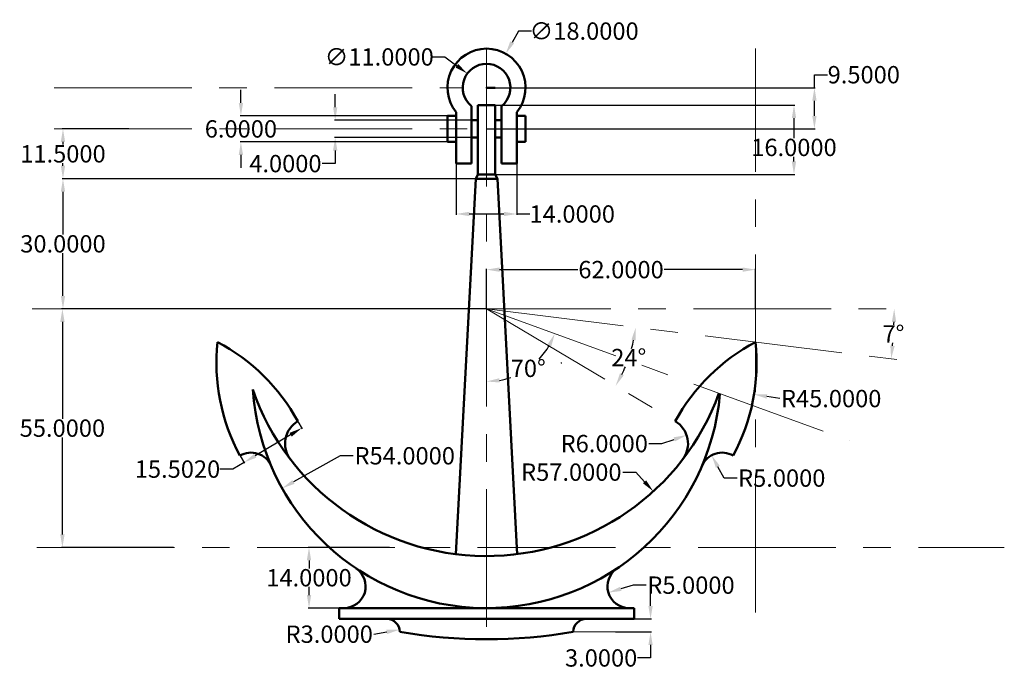
# Model space of a CAD drawing. Units: millimetres. Extents: x 434 to 661, y 625 to 775.
import ezdxf

# ---------------------------------------------------------------- set-up
doc = ezdxf.new("R2010")
doc.units = ezdxf.units.MM
doc.header["$MEASUREMENT"] = 0
doc.linetypes.add('CENTER', pattern=[50.8, 31.75, -6.35, 6.35, -6.35])
for name, color, linetype, lineweight in [('M-CNTR', 1, 'CENTER', 18), ('M-DIMS', 2, 'Continuous', 25), ('M-OUTL', 7, 'Continuous', 50)]:
    doc.layers.add(name, color=color, linetype=linetype, lineweight=lineweight)
doc.styles.get("Standard").update_dxf_attribs({"font": 'arial.ttf'})
doc.dimstyles.get("Standard").update_dxf_attribs({"dimtxt": 4, "dimasz": 3, "dimexe": 0.18, "dimexo": 0.0625, "dimgap": 0.09, "dimtad": 0, "dimtih": 1, "dimtoh": 1, "dimdec": 4, "dimzin": 0, "dimdsep": 46, "dimtxsty": 'Standard', "dimcen": 0.09, "dimadec": 0, "dimazin": 0, "dimtfac": 1, "dimtdec": 4, "dimtofl": 0, "dimtmove": 0, "dimatfit": 3, "dimfxl": 1, "dimtolj": 1, "dimtzin": 0, "dimarcsym": 0})

# ---------------------------------------------------------------- blocks, each defined once
blk = doc.blocks.new('*D1')
at = {"layer": 'Defpoints', "color": 0, "transparency": 16777216}
for p in [(558.86, 696.06), (603.27, 688.77)]:
    blk.add_point(p, dxfattribs=at)
at = {"layer": 'M-DIMS', "color": 0, "lineweight": -2, "transparency": 16777216}
for p, q in [((558.77, 696.06), (558.95, 696.06)), ((558.86, 695.97), (558.86, 696.15)), ((609.19, 687.8), (606.23, 688.28))]:
    blk.add_line(p, q, dxfattribs=at)
at = {"layer": 'M-DIMS', "color": 0, "transparency": 16777216}
blk.add_solid([(606.31, 688.78), (606.14, 687.79), (603.27, 688.77)], dxfattribs=at)
at = {"layer": 'M-DIMS', "color": 0, "transparency": 16777216, "insert": (621.04, 687.8), "char_height": 4, "attachment_point": 5}
blk.add_mtext('\\A1;R45.0000', dxfattribs=at)
blk = doc.blocks.new('*D2')
at = {"layer": 'Defpoints', "color": 0, "transparency": 16777216}
for p in [(593.47, 674.73), (595.87, 670.34)]:
    blk.add_point(p, dxfattribs=at)
at = {"layer": 'M-DIMS', "color": 0, "lineweight": -2, "transparency": 16777216}
for p, q in [((596.35, 669.47), (594.91, 672.1)), ((599.35, 669.47), (596.35, 669.47))]:
    blk.add_line(p, q, dxfattribs=at)
at = {"layer": 'M-DIMS', "color": 0, "transparency": 16777216}
blk.add_solid([(595.35, 672.34), (594.47, 671.86), (593.47, 674.73)], dxfattribs=at)
at = {"layer": 'M-DIMS', "color": 0, "transparency": 16777216, "insert": (609.65, 669.47), "char_height": 4, "attachment_point": 5}
blk.add_mtext('\\A1;R5.0000', dxfattribs=at)
blk = doc.blocks.new('*D3')
at = {"layer": 'Defpoints', "color": 0, "transparency": 16777216}
for p in [(587.72, 679.37), (582.04, 677.42)]:
    blk.add_point(p, dxfattribs=at)
at = {"layer": 'M-DIMS', "color": 0, "lineweight": -2, "transparency": 16777216}
for p, q in [((579.04, 677.42), (582.04, 677.42)), ((582.04, 677.42), (584.88, 678.39))]:
    blk.add_line(p, q, dxfattribs=at)
at = {"layer": 'M-DIMS', "color": 0, "transparency": 16777216}
blk.add_solid([(584.72, 678.87), (585.04, 677.92), (587.72, 679.37)], dxfattribs=at)
at = {"layer": 'M-DIMS', "color": 0, "transparency": 16777216, "insert": (568.74, 677.42), "char_height": 4, "attachment_point": 5}
blk.add_mtext('\\A1;R6.0000', dxfattribs=at)
blk = doc.blocks.new('*D4')
at = {"layer": 'Defpoints', "color": 0, "transparency": 16777216}
for p in [(541.61, 708.49), (580.05, 666.41)]:
    blk.add_point(p, dxfattribs=at)
at = {"layer": 'M-DIMS', "color": 0, "lineweight": -2, "transparency": 16777216}
for p, q in [((573, 670.84), (576, 670.84)), ((576, 670.84), (578.02, 668.62))]:
    blk.add_line(p, q, dxfattribs=at)
at = {"layer": 'M-DIMS', "color": 0, "transparency": 16777216}
blk.add_solid([(578.39, 668.96), (577.65, 668.28), (580.05, 666.41)], dxfattribs=at)
at = {"layer": 'M-DIMS', "color": 0, "transparency": 16777216, "insert": (561.15, 670.84), "char_height": 4, "attachment_point": 5}
blk.add_mtext('\\A1;R57.0000', dxfattribs=at)
blk = doc.blocks.new('*D5')
at = {"layer": 'Defpoints', "color": 0, "transparency": 16777216}
for p in [(541.61, 693.49), (494.49, 667.11)]:
    blk.add_point(p, dxfattribs=at)
at = {"layer": 'M-DIMS', "color": 0, "lineweight": -2, "transparency": 16777216}
for p, q in [((507.89, 674.61), (497.11, 668.57)), ((510.89, 674.61), (507.89, 674.61))]:
    blk.add_line(p, q, dxfattribs=at)
at = {"layer": 'M-DIMS', "color": 0, "transparency": 16777216}
blk.add_solid([(496.86, 669.01), (497.35, 668.14), (494.49, 667.11)], dxfattribs=at)
at = {"layer": 'M-DIMS', "color": 0, "transparency": 16777216, "insert": (522.75, 674.61), "char_height": 4, "attachment_point": 5}
blk.add_mtext('\\A1;R54.0000', dxfattribs=at)
blk = doc.blocks.new('*D6')
at = {"layer": 'Defpoints', "color": 0, "transparency": 16777216}
for p in [(569.68, 643.05), (574.47, 644.49)]:
    blk.add_point(p, dxfattribs=at)
at = {"layer": 'M-DIMS', "color": 0, "lineweight": -2, "transparency": 16777216}
for p, q in [((575.43, 644.78), (572.55, 643.92)), ((578.43, 644.78), (575.43, 644.78))]:
    blk.add_line(p, q, dxfattribs=at)
at = {"layer": 'M-DIMS', "color": 0, "transparency": 16777216}
blk.add_solid([(572.41, 644.4), (572.7, 643.44), (569.68, 643.05)], dxfattribs=at)
at = {"layer": 'M-DIMS', "color": 0, "transparency": 16777216, "insert": (588.73, 644.78), "char_height": 4, "attachment_point": 5}
blk.add_mtext('\\A1;R5.0000', dxfattribs=at)
blk = doc.blocks.new('*D7')
at = {"layer": 'Defpoints', "color": 0, "transparency": 16777216}
for p in [(518.61, 633.99), (521.56, 634.51)]:
    blk.add_point(p, dxfattribs=at)
at = {"layer": 'M-DIMS', "color": 0, "lineweight": -2, "transparency": 16777216}
blk.add_line((515.65, 633.47), (518.61, 633.99), dxfattribs=at)
at = {"layer": 'M-DIMS', "color": 0, "transparency": 16777216}
blk.add_solid([(518.52, 634.49), (518.69, 633.5), (521.56, 634.51)], dxfattribs=at)
at = {"layer": 'M-DIMS', "color": 0, "transparency": 16777216, "insert": (505.35, 633.47), "char_height": 4, "attachment_point": 5}
blk.add_mtext('\\A1;R3.0000', dxfattribs=at)
blk = doc.blocks.new('*D8')
at = {"layer": 'Defpoints', "color": 0, "transparency": 16777216}
for p in [(541.61, 768.49), (541.61, 708.49), (548.24, 693.11), (625.17, 678.11), (541.61, 633.99)]:
    blk.add_point(p, dxfattribs=at)
at = {"layer": 'M-DIMS', "color": 0, "lineweight": -2, "transparency": 16777216}
for start, end in [(316.2273, 329.7461), (280.2724, 289.5813)]:
    blk.add_arc((541.61, 708.49), 16.76, start, end, dxfattribs=at)
at = {"layer": 'M-DIMS', "color": 0, "transparency": 16777216}
for points in [[(555.63, 700.26), (556.53, 699.84), (557.35, 702.77)], [(544.64, 691.51), (544.55, 692.5), (541.61, 691.74)]]:
    blk.add_solid(points, dxfattribs=at)
at = {"layer": 'M-DIMS', "color": 0, "transparency": 16777216, "insert": (551.22, 694.77), "char_height": 4, "attachment_point": 5}
blk.add_mtext('\\A1;70°', dxfattribs=at)
blk = doc.blocks.new('*D9')
at = {"layer": 'Defpoints', "color": 0, "transparency": 16777216}
for p in [(436.88, 708.49), (541.61, 708.49), (639.54, 708.49), (635.25, 700.8), (639.75, 696.37)]:
    blk.add_point(p, dxfattribs=at)
at = {"layer": 'M-DIMS', "color": 0, "lineweight": -2, "transparency": 16777216}
for start, end in [(357.7555, 358.1705), (354.7882, 355.2015)]:
    blk.add_arc((541.61, 708.49), 93.96, start, end, dxfattribs=at)
at = {"layer": 'M-DIMS', "color": 0, "transparency": 16777216}
for points in [[(635.02, 705.5), (636.02, 705.49), (635.57, 708.49)], [(635.67, 699.91), (634.68, 700.01), (634.86, 696.98)]]:
    blk.add_solid(points, dxfattribs=at)
at = {"layer": 'M-DIMS', "color": 0, "transparency": 16777216, "insert": (635.39, 702.72), "char_height": 4, "attachment_point": 5}
blk.add_mtext('\\A1;7°', dxfattribs=at)
blk = doc.blocks.new('*D10')
at = {"layer": 'Defpoints', "color": 0, "transparency": 16777216}
for p in [(541.61, 708.49), (541.61, 708.49), (573.54, 695.02), (639.75, 696.37), (585.12, 682.57)]:
    blk.add_point(p, dxfattribs=at)
at = {"layer": 'M-DIMS', "color": 0, "lineweight": -2, "transparency": 16777216}
for start, end in [(344.7166, 347.9975), (334.1761, 337.3763)]:
    blk.add_arc((541.61, 708.49), 34.66, start, end, dxfattribs=at)
at = {"layer": 'M-DIMS', "color": 0, "transparency": 16777216}
for points in [[(575.01, 701.37), (576, 701.2), (576, 704.25)], [(573.24, 693.16), (572.36, 693.63), (571.38, 690.76)]]:
    blk.add_solid(points, dxfattribs=at)
at = {"layer": 'M-DIMS', "color": 0, "transparency": 16777216, "insert": (574.39, 697.26), "char_height": 4, "attachment_point": 5}
blk.add_mtext('\\A1;24°', dxfattribs=at)
blk = doc.blocks.new('*D11')
at = {"layer": 'Defpoints', "color": 0, "transparency": 16777216}
for p in [(603.61, 717.54), (541.61, 708.49), (603.61, 708.49)]:
    blk.add_point(p, dxfattribs=at)
at = {"layer": 'M-DIMS', "color": 0, "lineweight": -2, "transparency": 16777216}
for p, q in [((541.61, 708.56), (541.61, 717.72)), ((544.61, 717.54), (562.66, 717.54)), ((600.61, 717.54), (582.56, 717.54)), ((603.61, 708.56), (603.61, 717.72))]:
    blk.add_line(p, q, dxfattribs=at)
at = {"layer": 'M-DIMS', "color": 0, "transparency": 16777216}
for points in [[(544.61, 718.04), (544.61, 717.04), (541.61, 717.54)], [(600.61, 718.04), (600.61, 717.04), (603.61, 717.54)]]:
    blk.add_solid(points, dxfattribs=at)
at = {"layer": 'M-DIMS', "color": 0, "transparency": 16777216, "insert": (572.61, 717.54), "char_height": 4, "attachment_point": 5}
blk.add_mtext('\\A1;62.0000', dxfattribs=at)
blk = doc.blocks.new('*D12')
at = {"layer": 'Defpoints', "color": 0, "transparency": 16777216}
for p in [(519.28, 653.49), (500.69, 639.49), (519.28, 639.49)]:
    blk.add_point(p, dxfattribs=at)
at = {"layer": 'M-DIMS', "color": 0, "lineweight": -2, "transparency": 16777216}
for p, q in [((519.21, 653.49), (500.51, 653.49)), ((500.69, 650.49), (500.69, 648.63)), ((500.69, 642.49), (500.69, 644.36)), ((519.21, 639.49), (500.51, 639.49))]:
    blk.add_line(p, q, dxfattribs=at)
at = {"layer": 'M-DIMS', "color": 0, "transparency": 16777216}
for points in [[(500.19, 650.49), (501.19, 650.49), (500.69, 653.49)], [(500.19, 642.49), (501.19, 642.49), (500.69, 639.49)]]:
    blk.add_solid(points, dxfattribs=at)
at = {"layer": 'M-DIMS', "color": 0, "transparency": 16777216, "insert": (500.69, 646.49), "char_height": 4, "attachment_point": 5}
blk.add_mtext('\\A1;14.0000', dxfattribs=at)
blk = doc.blocks.new('*D13')
at = {"layer": 'Defpoints', "color": 0, "transparency": 16777216}
for p in [(571.27, 636.99), (571.27, 633.99), (579.41, 633.99)]:
    blk.add_point(p, dxfattribs=at)
at = {"layer": 'M-DIMS', "color": 0, "lineweight": -2, "transparency": 16777216}
for p, q in [((579.41, 639.99), (579.41, 642.99)), ((571.33, 636.99), (579.59, 636.99)), ((571.33, 633.99), (579.59, 633.99)), ((579.41, 630.99), (579.41, 627.99)), ((579.41, 627.99), (576.41, 627.99))]:
    blk.add_line(p, q, dxfattribs=at)
at = {"layer": 'M-DIMS', "color": 0, "transparency": 16777216}
for points in [[(578.91, 639.99), (579.91, 639.99), (579.41, 636.99)], [(578.91, 630.99), (579.91, 630.99), (579.41, 633.99)]]:
    blk.add_solid(points, dxfattribs=at)
at = {"layer": 'M-DIMS', "color": 0, "transparency": 16777216, "insert": (568.02, 627.99), "char_height": 4, "attachment_point": 5}
blk.add_mtext('\\A1;3.0000', dxfattribs=at)
blk = doc.blocks.new('*D14')
at = {"layer": 'Defpoints', "color": 0, "transparency": 16777216}
for p in [(443.85, 708.49), (469.53, 708.49), (469.53, 653.49)]:
    blk.add_point(p, dxfattribs=at)
at = {"layer": 'M-DIMS', "color": 0, "lineweight": -2, "transparency": 16777216}
for p, q in [((469.47, 708.49), (443.67, 708.49)), ((443.85, 705.49), (443.85, 683.13)), ((443.85, 656.49), (443.85, 678.86)), ((469.47, 653.49), (443.67, 653.49))]:
    blk.add_line(p, q, dxfattribs=at)
at = {"layer": 'M-DIMS', "color": 0, "transparency": 16777216}
for points in [[(443.35, 705.49), (444.35, 705.49), (443.85, 708.49)], [(443.35, 656.49), (444.35, 656.49), (443.85, 653.49)]]:
    blk.add_solid(points, dxfattribs=at)
at = {"layer": 'M-DIMS', "color": 0, "transparency": 16777216, "insert": (443.85, 680.99), "char_height": 4, "attachment_point": 5}
blk.add_mtext('\\A1;55.0000', dxfattribs=at)
blk = doc.blocks.new('*D15')
at = {"layer": 'Defpoints', "color": 0, "transparency": 16777216}
for p in [(443.98, 738.49), (541.61, 738.49), (541.61, 708.49)]:
    blk.add_point(p, dxfattribs=at)
at = {"layer": 'M-DIMS', "color": 0, "lineweight": -2, "transparency": 16777216}
for p, q in [((541.54, 738.49), (443.8, 738.49)), ((443.98, 735.49), (443.98, 725.63)), ((443.98, 711.49), (443.98, 721.36)), ((541.54, 708.49), (443.8, 708.49))]:
    blk.add_line(p, q, dxfattribs=at)
at = {"layer": 'M-DIMS', "color": 0, "transparency": 16777216}
for points in [[(443.48, 735.49), (444.48, 735.49), (443.98, 738.49)], [(443.48, 711.49), (444.48, 711.49), (443.98, 708.49)]]:
    blk.add_solid(points, dxfattribs=at)
at = {"layer": 'M-DIMS', "color": 0, "transparency": 16777216, "insert": (443.98, 723.49), "char_height": 4, "attachment_point": 5}
blk.add_mtext('\\A1;30.0000', dxfattribs=at)
blk = doc.blocks.new('*D16')
at = {"layer": 'Defpoints', "color": 0, "transparency": 16777216}
for p in [(459.2, 749.99), (443.98, 738.49), (459.2, 738.49)]:
    blk.add_point(p, dxfattribs=at)
at = {"layer": 'M-DIMS', "color": 0, "lineweight": -2, "transparency": 16777216}
for p, q in [((459.14, 749.99), (443.8, 749.99)), ((443.98, 746.99), (443.98, 746.38)), ((443.98, 741.49), (443.98, 742.11)), ((459.14, 738.49), (443.8, 738.49))]:
    blk.add_line(p, q, dxfattribs=at)
at = {"layer": 'M-DIMS', "color": 0, "transparency": 16777216}
for points in [[(443.48, 746.99), (444.48, 746.99), (443.98, 749.99)], [(443.48, 741.49), (444.48, 741.49), (443.98, 738.49)]]:
    blk.add_solid(points, dxfattribs=at)
at = {"layer": 'M-DIMS', "color": 0, "transparency": 16777216, "insert": (443.98, 744.24), "char_height": 4, "attachment_point": 5}
blk.add_mtext('\\A1;11.5000', dxfattribs=at)
blk = doc.blocks.new('*D17')
at = {"layer": 'Defpoints', "color": 0, "transparency": 16777216}
for p in [(541.61, 759.49), (617.18, 759.49), (541.61, 749.99)]:
    blk.add_point(p, dxfattribs=at)
at = {"layer": 'M-DIMS', "color": 0, "lineweight": -2, "transparency": 16777216}
for p, q in [((617.18, 759.49), (617.18, 762.49)), ((617.18, 762.49), (620.18, 762.49)), ((541.67, 759.49), (617.36, 759.49)), ((617.18, 752.99), (617.18, 756.49)), ((541.67, 749.99), (617.36, 749.99))]:
    blk.add_line(p, q, dxfattribs=at)
at = {"layer": 'M-DIMS', "color": 0, "transparency": 16777216}
for points in [[(616.68, 756.49), (617.68, 756.49), (617.18, 759.49)], [(616.68, 752.99), (617.68, 752.99), (617.18, 749.99)]]:
    blk.add_solid(points, dxfattribs=at)
at = {"layer": 'M-DIMS', "color": 0, "transparency": 16777216, "insert": (628.56, 762.49), "char_height": 4, "attachment_point": 5}
blk.add_mtext('\\A1;9.5000', dxfattribs=at)
blk = doc.blocks.new('*D18')
at = {"layer": 'Defpoints', "color": 0, "transparency": 16777216}
for p in [(546.03, 767.33), (537.18, 751.66)]:
    blk.add_point(p, dxfattribs=at)
at = {"layer": 'M-DIMS', "color": 0, "lineweight": -2, "transparency": 16777216}
for p, q in [((548.99, 772.55), (547.51, 769.94)), ((551.99, 772.55), (548.99, 772.55)), ((541.52, 759.49), (541.7, 759.49)), ((541.61, 759.4), (541.61, 759.58))]:
    blk.add_line(p, q, dxfattribs=at)
at = {"layer": 'M-DIMS', "color": 0, "transparency": 16777216}
blk.add_solid([(547.07, 770.19), (547.95, 769.69), (546.03, 767.33)], dxfattribs=at)
at = {"layer": 'M-DIMS', "color": 0, "transparency": 16777216, "insert": (564.1, 772.55), "char_height": 4, "attachment_point": 5}
blk.add_mtext('\\A1;∅18.0000', dxfattribs=at)
blk = doc.blocks.new('*D19')
at = {"layer": 'Defpoints', "color": 0, "transparency": 16777216}
for p in [(537.18, 762.76), (546.03, 756.23)]:
    blk.add_point(p, dxfattribs=at)
at = {"layer": 'M-DIMS', "color": 0, "lineweight": -2, "transparency": 16777216}
for p, q in [((529, 766.59), (532, 766.59)), ((532, 766.59), (534.77, 764.54)), ((541.52, 759.49), (541.7, 759.49)), ((541.61, 759.4), (541.61, 759.58))]:
    blk.add_line(p, q, dxfattribs=at)
at = {"layer": 'M-DIMS', "color": 0, "transparency": 16777216}
blk.add_solid([(535.07, 764.95), (534.47, 764.14), (537.18, 762.76)], dxfattribs=at)
at = {"layer": 'M-DIMS', "color": 0, "transparency": 16777216, "insert": (516.88, 766.59), "char_height": 4, "attachment_point": 5}
blk.add_mtext('\\A1;∅11.0000', dxfattribs=at)
blk = doc.blocks.new('*D20')
at = {"layer": 'Defpoints', "color": 0, "transparency": 16777216}
for p in [(542.91, 755.49), (542.91, 739.49), (612.47, 739.49)]:
    blk.add_point(p, dxfattribs=at)
at = {"layer": 'M-DIMS', "color": 0, "lineweight": -2, "transparency": 16777216}
for p, q in [((542.97, 755.49), (612.65, 755.49)), ((612.47, 752.49), (612.47, 747.85)), ((612.47, 742.49), (612.47, 743.58)), ((542.97, 739.49), (612.65, 739.49))]:
    blk.add_line(p, q, dxfattribs=at)
at = {"layer": 'M-DIMS', "color": 0, "transparency": 16777216}
for points in [[(611.97, 752.49), (612.97, 752.49), (612.47, 755.49)], [(611.97, 742.49), (612.97, 742.49), (612.47, 739.49)]]:
    blk.add_solid(points, dxfattribs=at)
at = {"layer": 'M-DIMS', "color": 0, "transparency": 16777216, "insert": (612.47, 745.72), "char_height": 4, "attachment_point": 5}
blk.add_mtext('\\A1;16.0000', dxfattribs=at)
blk = doc.blocks.new('*D21')
at = {"layer": 'Defpoints', "color": 0, "transparency": 16777216}
for p in [(532.61, 752.99), (484.99, 746.99), (532.61, 746.99)]:
    blk.add_point(p, dxfattribs=at)
at = {"layer": 'M-DIMS', "color": 0, "lineweight": -2, "transparency": 16777216}
for p, q in [((484.99, 755.99), (484.99, 758.99)), ((532.54, 752.99), (484.81, 752.99)), ((532.54, 746.99), (484.81, 746.99)), ((484.99, 743.99), (484.99, 740.99))]:
    blk.add_line(p, q, dxfattribs=at)
at = {"layer": 'M-DIMS', "color": 0, "transparency": 16777216}
for points in [[(484.49, 755.99), (485.49, 755.99), (484.99, 752.99)], [(484.49, 743.99), (485.49, 743.99), (484.99, 746.99)]]:
    blk.add_solid(points, dxfattribs=at)
at = {"layer": 'M-DIMS', "color": 0, "transparency": 16777216, "insert": (484.99, 749.99), "char_height": 4, "attachment_point": 5}
blk.add_mtext('\\A1;6.0000', dxfattribs=at)
blk = doc.blocks.new('*D22')
at = {"layer": 'Defpoints', "color": 0, "transparency": 16777216}
for p in [(539.16, 751.99), (506.72, 747.99), (539.16, 747.99)]:
    blk.add_point(p, dxfattribs=at)
at = {"layer": 'M-DIMS', "color": 0, "lineweight": -2, "transparency": 16777216}
for p, q in [((506.72, 754.99), (506.72, 757.99)), ((539.1, 751.99), (506.54, 751.99)), ((539.1, 747.99), (506.54, 747.99)), ((506.72, 744.99), (506.72, 741.99)), ((506.72, 741.99), (503.72, 741.99))]:
    blk.add_line(p, q, dxfattribs=at)
at = {"layer": 'M-DIMS', "color": 0, "transparency": 16777216}
for points in [[(506.22, 754.99), (507.22, 754.99), (506.72, 751.99)], [(506.22, 744.99), (507.22, 744.99), (506.72, 747.99)]]:
    blk.add_solid(points, dxfattribs=at)
at = {"layer": 'M-DIMS', "color": 0, "transparency": 16777216, "insert": (495.25, 741.99), "char_height": 4, "attachment_point": 5}
blk.add_mtext('\\A1;4.0000', dxfattribs=at)
blk = doc.blocks.new('*D23')
at = {"layer": 'Defpoints', "color": 0, "transparency": 16777216}
for p in [(534.61, 741.99), (548.61, 741.99), (548.61, 730.37)]:
    blk.add_point(p, dxfattribs=at)
at = {"layer": 'M-DIMS', "color": 0, "lineweight": -2, "transparency": 16777216}
for p, q in [((534.61, 741.93), (534.61, 730.19)), ((548.61, 741.93), (548.61, 730.19)), ((537.61, 730.37), (545.61, 730.37)), ((548.61, 730.37), (551.61, 730.37))]:
    blk.add_line(p, q, dxfattribs=at)
at = {"layer": 'M-DIMS', "color": 0, "transparency": 16777216}
for points in [[(537.61, 730.87), (537.61, 729.87), (534.61, 730.37)], [(545.61, 730.87), (545.61, 729.87), (548.61, 730.37)]]:
    blk.add_solid(points, dxfattribs=at)
at = {"layer": 'M-DIMS', "color": 0, "transparency": 16777216, "insert": (561.36, 730.37), "char_height": 4, "attachment_point": 5}
blk.add_mtext('\\A1;14.0000', dxfattribs=at)
blk = doc.blocks.new('*D24')
at = {"layer": 'Defpoints', "color": 0, "transparency": 16777216}
for p in [(498.1, 682.57), (484.78, 674.64), (485.71, 673.07)]:
    blk.add_point(p, dxfattribs=at)
at = {"layer": 'M-DIMS', "color": 0, "lineweight": -2, "transparency": 16777216}
for p, q in [((498.13, 682.52), (499.12, 680.85)), ((496.45, 679.47), (488.29, 674.61)), ((484.81, 674.58), (485.8, 672.92)), ((485.71, 673.07), (483.13, 671.54)), ((483.13, 671.54), (480.13, 671.54))]:
    blk.add_line(p, q, dxfattribs=at)
at = {"layer": 'M-DIMS', "color": 0, "transparency": 16777216}
for points in [[(496.2, 679.9), (496.71, 679.04), (499.03, 681.01)], [(488.03, 675.04), (488.55, 674.18), (485.71, 673.07)]]:
    blk.add_solid(points, dxfattribs=at)
at = {"layer": 'M-DIMS', "color": 0, "transparency": 16777216, "insert": (470.38, 671.54), "char_height": 4, "attachment_point": 5}
blk.add_mtext('\\A1;15.5020', dxfattribs=at)

msp = doc.modelspace()

# ---------------------------------------------------------------- linework, layer by layer
at = {"layer": 'M-CNTR'}
for p, q in [((541.60596, 768.49348), (541.60596, 633.99348)), ((603.60596, 638.49348), (603.60596, 768.49348)), ((441.91855, 759.49348), (536.10596, 759.49348)), ((441.92581, 749.99348), (543.60596, 749.99348)), ((436.87638, 708.49348), (639.54354, 708.49348)), ((541.60596, 708.49348), (625.16702, 678.11024)), ((541.60596, 708.49348), (639.74583, 696.37165)), ((541.60596, 708.49348), (585.1154, 682.57189)), ((437.94776, 653.49348), (660.9457, 653.49348)), ((575.60596, 633.99348), (561.60596, 633.99348))]:
    msp.add_line(p, q, dxfattribs=at)
at = {"layer": 'M-OUTL'}
for p, q in [((541.60596, 759.49348), (543.60596, 759.49348)), ((534.60596, 753.83662), (534.60596, 741.99348)), ((538.12398, 755.23603), (538.12398, 741.99348)), ((539.60596, 755.49348), (539.60596, 739.49348)), ((539.60596, 755.49348), (543.60596, 755.49348)), ((543.60596, 755.49348), (543.60596, 739.49348)), ((545.08794, 755.23603), (545.08794, 741.99348)), ((548.60596, 753.83662), (548.60596, 741.99348)), ((532.60596, 752.99348), (534.60596, 752.99348)), ((532.60596, 752.99348), (532.60596, 746.99348)), ((538.12398, 751.99348), (539.60596, 751.99348)), ((545.08794, 751.99348), (543.60596, 751.99348)), ((548.60596, 752.99348), (550.60596, 752.99348)), ((550.60596, 752.99348), (550.60596, 746.99348)), ((532.60596, 746.99348), (534.60596, 746.99348)), ((538.12398, 747.99348), (539.60596, 747.99348)), ((545.08794, 747.99348), (543.60596, 747.99348)), ((548.60596, 746.99348), (550.60596, 746.99348)), ((534.60596, 741.99348), (538.12398, 741.99348)), ((548.60596, 741.99348), (545.08794, 741.99348)), ((534.52346, 651.9352), (539.10384, 738.45352)), ((539.10384, 738.45352), (539.60596, 739.49348)), ((539.10596, 738.49348), (544.10596, 738.49348)), ((539.60596, 739.49348), (543.60596, 739.49348)), ((544.10596, 738.49348), (543.60596, 739.49348)), ((548.68846, 651.9352), (544.10596, 738.49348)), ((507.60596, 639.49348), (575.60596, 639.49348)), ((507.60596, 636.99348), (507.60596, 639.49348)), ((575.60596, 639.49348), (575.60596, 636.99348)), ((575.60596, 636.99348), (507.60596, 636.99348))]:
    msp.add_line(p, q, dxfattribs=at)
for centre, radius, start, end in [((541.60596, 759.49348), 9, 90, 218.9424413), ((541.60596, 759.49348), 9, 321.0575587, 90), ((541.60596, 759.49348), 5.5, 90, 230.7217931), ((541.60596, 759.49348), 5.5, 309.2782069, 90), ((524.35197, 696.06116), 45, 173.9096643, 208.4295853), ((458.57573, 661.05196), 45, 28.5692553, 62.1383344), ((624.63619, 661.05196), 45, 117.8616656, 151.4307447), ((558.85995, 696.06116), 45, 331.5704147, 6.0903357), ((541.60596, 708.49348), 57, 199.0453108, 340.01847), ((541.60596, 693.49348), 54, 183.8225537, 355.1512209), ((501.16744, 677.41734), 6, 120.7851817, 217.5415087), ((582.04448, 677.41734), 6, 322.4584913, 59.2148183), ((487.33795, 670.34217), 5, 23.1036048, 120.7851817), ((595.87397, 670.34217), 5, 59.2148183, 156.8963952), ((508.74261, 644.49348), 5, 270, 56.1510061), ((574.46931, 644.49348), 5, 123.8489939, 270), ((518.60596, 633.99348), 3, 0, 90), ((564.60596, 633.99348), 3, 90, 180), ((541.60596, 751.32625), 119.02513, 260.3265997, 279.6734003)]:
    msp.add_arc(centre, radius, start, end, dxfattribs=at)

# ---------------------------------------------------------------- dimensions: what is measured, and where the dimension line sits
at = {"layer": 'M-DIMS'}
dim = msp.add_diameter_dim_2p(p1=(537.17771, 751.65826), p2=(546.03421, 767.32869), dimstyle='Standard', override={"dimclrd": 0, "dimclre": 0, "dimclrt": 0}, dxfattribs=at)
dim.commit()
dim.dimension.update_dxf_attribs({"geometry": '*D18', "text_midpoint": (564.10229, 772.55217)})
dim = msp.add_diameter_dim_2p(p1=(546.03012, 756.22594), p2=(537.1818, 762.76101), dimstyle='Standard', override={"dimclrd": 0, "dimclre": 0, "dimclrt": 0}, dxfattribs=at)
dim.commit()
dim.dimension.update_dxf_attribs({"geometry": '*D19', "text_midpoint": (516.88045, 766.5908), "dimtype": 163})
for base, line1, line2, picture, middle in [((548.24409, 693.10911), ((541.60596, 708.49348), (625.16702, 678.11024)), ((541.60596, 768.49348), (541.60596, 633.99348)), '*D8', (551.21867, 694.7698)), ((635.24992, 700.80411), ((541.60596, 708.49348), (639.74583, 696.37165)), ((436.87638, 708.49348), (639.54354, 708.49348)), '*D9', (635.38776, 702.72363)), ((573.53826, 695.02409), ((541.60596, 708.49348), (639.74583, 696.37165)), ((541.60596, 708.49348), (585.1154, 682.57189)), '*D10', (574.39169, 697.25995))]:
    dim = msp.add_angular_dim_2l(base=base, line1=line1, line2=line2, dimstyle='Standard', override={"dimclrd": 0, "dimclre": 0, "dimclrt": 0}, dxfattribs=at)
    dim.commit()
    dim.dimension.update_dxf_attribs({"geometry": picture, "text_midpoint": middle})
for base, p1, p2, picture, middle in [((617.17762, 759.49348), (541.60596, 749.99348), (541.60596, 759.49348), '*D17', (628.56366, 762.49348)), ((506.72054, 747.99348), (539.16301, 751.99348), (539.16301, 747.99348), '*D22', (495.25401, 741.99348)), ((443.9823, 738.49348), (459.19929, 749.99348), (459.19929, 738.49348), '*D16', (443.9823, 744.24348)), ((443.9823, 738.49348), (541.60596, 708.49348), (541.60596, 738.49348), '*D15', (443.9823, 723.49348)), ((443.84854, 708.49348), (469.52929, 653.49348), (469.52929, 708.49348), '*D14', (443.84854, 680.99348)), ((500.69498, 639.49348), (519.27667, 653.49348), (519.27667, 639.49348), '*D12', (500.69498, 646.49348)), ((579.40782, 633.99348), (571.26802, 636.99348), (571.26802, 633.99348), '*D13', (568.02314, 627.99348))]:
    dim = msp.add_linear_dim(base=base, p1=p1, p2=p2, angle=90, dimstyle='Standard', override={"dimclrd": 0, "dimclre": 0, "dimclrt": 0}, dxfattribs=at)
    dim.commit()
    dim.dimension.update_dxf_attribs({"geometry": picture, "text_midpoint": middle})
for base, p1, p2, picture, middle in [((484.98944, 746.99348), (532.60596, 752.99348), (532.60596, 746.99348), '*D21', (484.98944, 749.99348)), ((612.46937, 739.49348), (542.90838, 755.49348), (542.90838, 739.49348), '*D20', (612.46937, 745.71535))]:
    dim = msp.add_linear_dim(base=base, p1=p1, p2=p2, angle=90, dimstyle='Standard', override={"dimclrd": 0, "dimclre": 0, "dimclrt": 0}, dxfattribs=at)
    dim.commit()
    dim.dimension.update_dxf_attribs({"geometry": picture, "text_midpoint": middle, "dimtype": 160})
for base, p1, p2, picture, middle in [((548.60596, 730.37111), (534.60596, 741.99348), (548.60596, 741.99348), '*D23', (561.35762, 730.37111)), ((603.60596, 717.54436), (541.60596, 708.49348), (603.60596, 708.49348), '*D11', (572.60596, 717.54436))]:
    dim = msp.add_linear_dim(base=base, p1=p1, p2=p2, dimstyle='Standard', override={"dimclrd": 0, "dimclre": 0, "dimclrt": 0}, dxfattribs=at)
    dim.commit()
    dim.dimension.update_dxf_attribs({"geometry": picture, "text_midpoint": middle})
for center, mpoint, picture, middle in [((541.60596, 708.49348), (580.04645, 666.40632), '*D4', (561.1461, 670.83655)), ((541.60596, 693.49348), (494.49186, 667.10671), '*D5', (522.74525, 674.6112)), ((582.04448, 677.41734), (587.7187, 679.36751), '*D3', (568.74438, 677.41734)), ((595.87397, 670.34217), (593.47276, 674.72785), '*D2', (609.65431, 669.46504)), ((574.46931, 644.49348), (569.68104, 643.05389), '*D6', (588.72706, 644.78139)), ((518.60596, 633.99348), (521.56072, 634.51253), '*D7', (515.6512, 633.47442))]:
    dim = msp.add_radius_dim(center=center, mpoint=mpoint, dimstyle='Standard', override={"dimclrd": 0, "dimclre": 0, "dimclrt": 0}, dxfattribs=at)
    dim.commit()
    dim.dimension.update_dxf_attribs({"geometry": picture, "text_midpoint": middle, "dimtype": 164})
dim = msp.add_radius_dim(center=(558.85995, 696.06116), mpoint=(603.26535, 688.77004), dimstyle='Standard', override={"dimclrd": 0, "dimclre": 0, "dimclrt": 0}, dxfattribs=at)
dim.commit()
dim.dimension.update_dxf_attribs({"geometry": '*D1', "text_midpoint": (621.04005, 687.79789)})
dim = msp.add_aligned_dim(p1=(498.09652, 682.57189), p2=(484.77884, 674.63763), distance=1.82313, dimstyle='Standard', override={"dimclrd": 0, "dimclre": 0, "dimclrt": 0}, dxfattribs=at)
dim.commit()
dim.dimension.update_dxf_attribs({"geometry": '*D24', "text_midpoint": (470.38302, 671.53593)})

doc.saveas('drawing.dxf')
